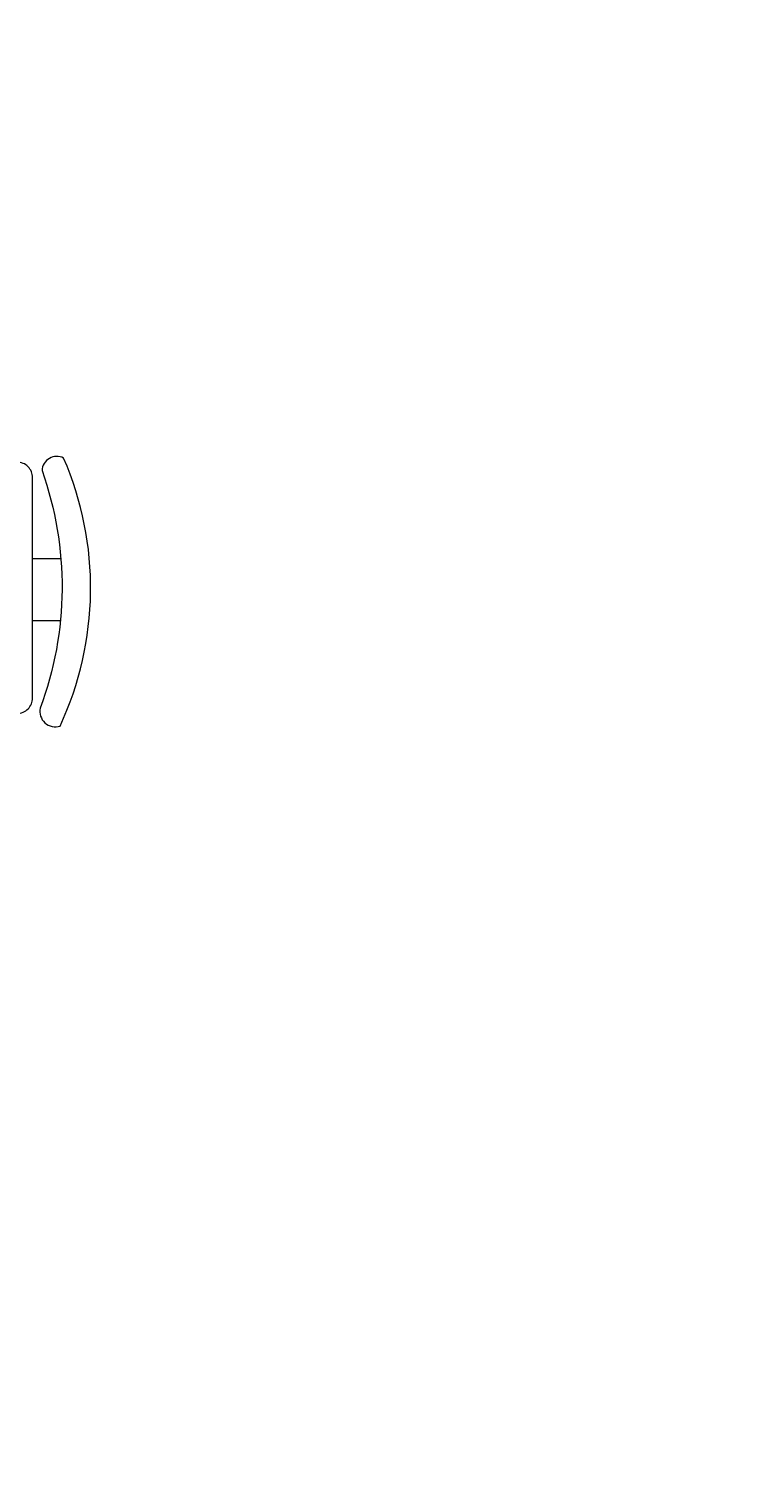
# Model space of a CAD drawing. Units: inches. Extents: x 1088 to 1703, y 668 to 1875.
# Tile 22 of 45: x 1413 to 1436, y 1623 to 1672. Entities that reach past the tile are written whole.
import ezdxf

# ---------------------------------------------------------------- set-up
doc = ezdxf.new("R2010")
doc.units = ezdxf.units.IN
doc.layers.add('A-ANNO-DIMS', color=2, linetype='Continuous', lineweight=18)
doc.layers.add('A-FURN', color=8, linetype='Continuous', lineweight=13)
doc.styles.get("Standard").update_dxf_attribs({"font": 'arial.ttf'})
doc.dimstyles.get("Standard").update_dxf_attribs({"dimtxt": 0.18, "dimasz": 0.18, "dimexe": 0.18, "dimexo": 0.0625, "dimgap": 0.09, "dimtad": 0, "dimtih": 1, "dimtoh": 1, "dimdec": 4, "dimzin": 0, "dimdsep": 46, "dimtxsty": 'Standard', "dimcen": 0.09, "dimadec": 0, "dimazin": 0, "dimtfac": 1, "dimtdec": 4, "dimtofl": 0, "dimtmove": 0, "dimatfit": 3, "dimfxl": 1, "dimtolj": 1, "dimtzin": 0, "dimarcsym": 0})

# ---------------------------------------------------------------- blocks, each defined once
blk = doc.blocks.new('*D38')
at = {"layer": 'A-ANNO-DIMS', "color": 0, "lineweight": -2, "transparency": 16777216}
for p, q in [((1317.345, 1736.945), (1317.345, 725.549)), ((1437.345, 1736.945), (1437.345, 725.549)), ((1317.525, 725.729), (1377.065, 725.729)), ((1437.165, 725.729), (1377.625, 725.729))]:
    blk.add_line(p, q, dxfattribs=at)
at = {"layer": 'A-ANNO-DIMS', "color": 0, "transparency": 16777216}
for points in [[(1317.525, 725.759), (1317.525, 725.699), (1317.345, 725.729)], [(1437.165, 725.759), (1437.165, 725.699), (1437.345, 725.729)]]:
    blk.add_solid(points, dxfattribs=at)
at = {"layer": 'Defpoints', "color": 0, "transparency": 16777216}
for p in [(1317.345, 1737.007), (1437.345, 1737.007), (1437.345, 725.729)]:
    blk.add_point(p, dxfattribs=at)
at = {"layer": 'A-ANNO-DIMS', "color": 0, "transparency": 16777216, "insert": (1377.345, 725.729), "char_height": 0.18, "attachment_point": 5}
blk.add_mtext('\\A1;120', dxfattribs=at)

msp = doc.modelspace()

# ---------------------------------------------------------------- linework, layer by layer
at = {"layer": 'A-FURN'}
for points in [[(1413.01, 1657.168, -0.175809), (1412.95, 1649.266, 0.578392), (1413.608, 1648.667, 0.214524), (1413.728, 1657.587, 0.552014), (1413.01, 1657.168, -0.065079)], [(1412.693, 1656.937, 0.414214), (1412.18, 1657.45), (1405.435, 1657.45, 0.414214), (1404.921, 1656.937), (1404.921, 1649.601, 0.414214), (1405.435, 1649.088), (1412.18, 1649.088, 0.414214), (1412.693, 1649.601), (1412.693, 1656.937)], [(1412.693, 1652.178), (1413.621, 1652.178, -0.064759)]]:
    msp.add_lwpolyline(points, format="xyb", dxfattribs=at)
msp.add_lwpolyline([(1413.637, 1654.231), (1412.693, 1654.231)], dxfattribs=at)

# ---------------------------------------------------------------- dimensions: what is measured, and where the dimension line sits
at = {"layer": 'A-ANNO-DIMS'}
dim = msp.add_linear_dim(base=(1437.345, 725.729), p1=(1317.345, 1737.007), p2=(1437.345, 1737.007), dimstyle='Standard', override={"dimdec": 0, "dimlfac": 1, "dimrnd": 0, "dimzin": 0, "dimdsep": 46, "dimlunit": 2}, dxfattribs=at)
dim.commit()
dim.dimension.update_dxf_attribs({"geometry": '*D38', "text_midpoint": (1377.345, 725.729)})

doc.saveas('drawing.dxf')
